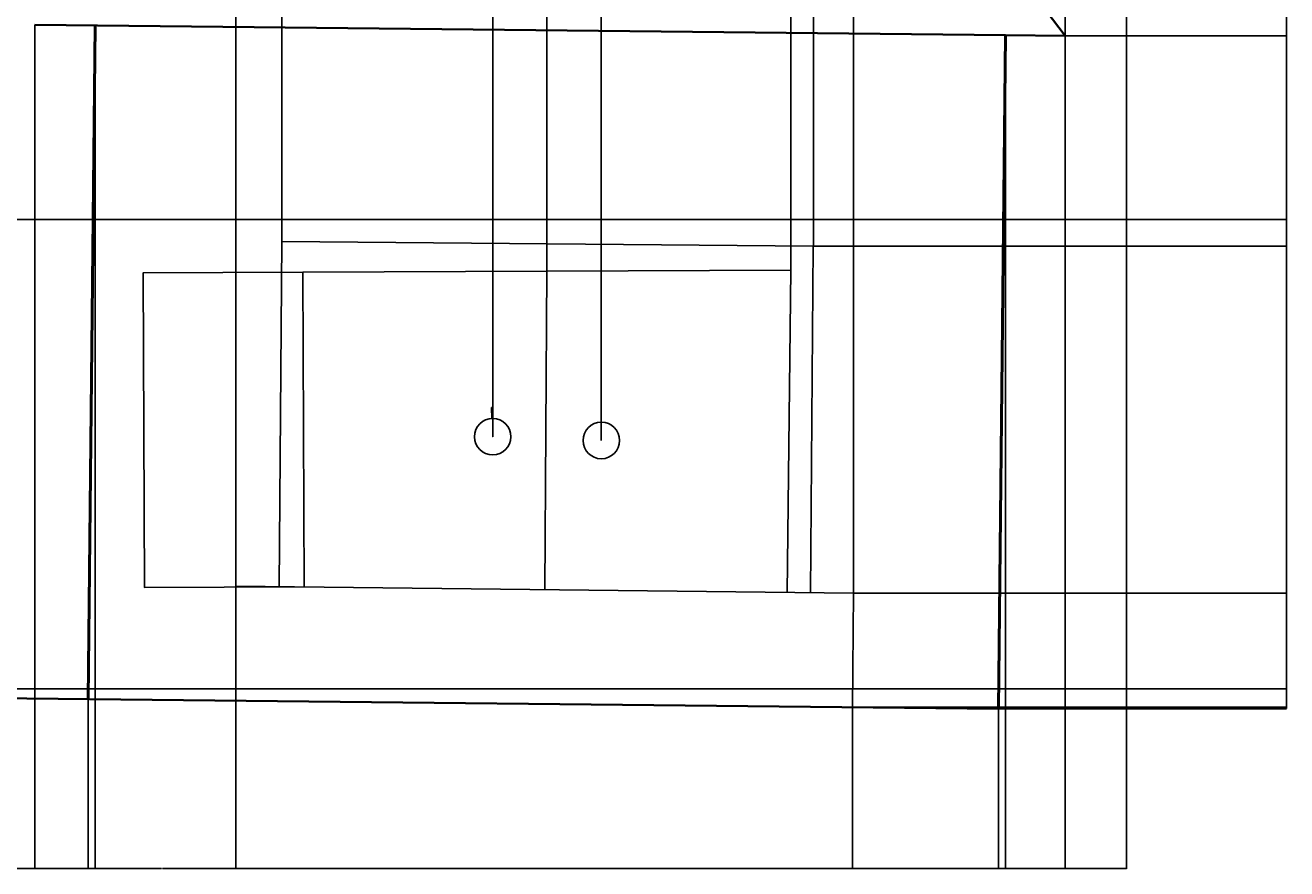
# Model space of a CAD drawing. Units: millimetres. Extents: x 1119 to 4262, y 854 to 2737.
# Tile 4 of 5: x 3118 to 4262, y 854 to 1620. Entities that reach past the tile are written whole.
import ezdxf

# ---------------------------------------------------------------- set-up
doc = ezdxf.new("R2010")
doc.units = ezdxf.units.MM
for name, color, linetype, lineweight in [('A-ANNO-DIMS', 2, 'Continuous', 18), ('A-DOOR', 3, 'Continuous', 25), ('A-ELEV', 8, 'Continuous', 35), ('A-FLOR-STRS', 6, 'Continuous', 25), ('A-ROOF', 1, 'Continuous', 35), ('A-WALL', 7, 'Continuous', 50)]:
    doc.layers.add(name, color=color, linetype=linetype, lineweight=lineweight)
doc.styles.get("Standard").update_dxf_attribs({"font": 'arial.ttf'})
doc.dimstyles.get("Standard").update_dxf_attribs({"dimtxt": 0.18, "dimasz": 0.18, "dimexe": 0.18, "dimexo": 0.0625, "dimgap": 0.09, "dimtad": 0, "dimtih": 1, "dimtoh": 1, "dimdec": 4, "dimzin": 0, "dimdsep": 46, "dimtxsty": 'Standard', "dimcen": 0.09, "dimadec": 0, "dimazin": 0, "dimtfac": 1, "dimtdec": 4, "dimtofl": 0, "dimtmove": 0, "dimatfit": 3, "dimfxl": 1, "dimtolj": 1, "dimtzin": 0, "dimarcsym": 0})

# ---------------------------------------------------------------- blocks, each defined once
blk = doc.blocks.new('*D9')
at = {"layer": 'A-ANNO-DIMS', "color": 0, "lineweight": -2, "transparency": 16777216}
for p, q in [((3099.2, 1180.2), (3099.2, 854.2)), ((3174.6, 1008), (3174.6, 854.2)), ((3099.4, 854.4), (3136.5, 854.4)), ((3174.4, 854.4), (3137.3, 854.4))]:
    blk.add_line(p, q, dxfattribs=at)
at = {"layer": 'A-ANNO-DIMS', "color": 0, "transparency": 16777216}
for points in [[(3099.4, 854.4), (3099.4, 854.3), (3099.2, 854.4)], [(3174.4, 854.4), (3174.4, 854.3), (3174.6, 854.4)]]:
    blk.add_solid(points, dxfattribs=at)
at = {"layer": 'Defpoints', "color": 0, "transparency": 16777216}
for p in [(3099.2, 1180.2), (3174.6, 1008.1), (3174.6, 854.4)]:
    blk.add_point(p, dxfattribs=at)
at = {"layer": 'A-ANNO-DIMS', "color": 0, "transparency": 16777216, "insert": (3136.9, 854.4), "char_height": 0.18, "attachment_point": 5}
blk.add_mtext('\\A1;75.38', dxfattribs=at)
blk = doc.blocks.new('*D10')
at = {"layer": 'A-ANNO-DIMS', "color": 0, "lineweight": -2, "transparency": 16777216}
for p, q in [((3174.6, 1008), (3174.6, 854.2)), ((3308.7, 1006.6), (3308.7, 854.2)), ((3174.7, 854.4), (3241.2, 854.4)), ((3308.5, 854.4), (3242.1, 854.4))]:
    blk.add_line(p, q, dxfattribs=at)
at = {"layer": 'A-ANNO-DIMS', "color": 0, "transparency": 16777216}
for points in [[(3174.7, 854.4), (3174.7, 854.3), (3174.6, 854.4)], [(3308.5, 854.4), (3308.5, 854.3), (3308.7, 854.4)]]:
    blk.add_solid(points, dxfattribs=at)
at = {"layer": 'Defpoints', "color": 0, "transparency": 16777216}
for p in [(3174.6, 1008.1), (3308.7, 1006.7), (3308.7, 854.4)]:
    blk.add_point(p, dxfattribs=at)
at = {"layer": 'A-ANNO-DIMS', "color": 0, "transparency": 16777216, "insert": (3241.6, 854.4), "char_height": 0.18, "attachment_point": 5}
blk.add_mtext('\\A1;134.12', dxfattribs=at)
blk = doc.blocks.new('*D11')
at = {"layer": 'A-ANNO-DIMS', "color": 0, "lineweight": -2, "transparency": 16777216}
for p, q in [((3308.7, 1006.6), (3308.7, 854.2)), ((4000.5, 999.3), (4000.5, 854.2)), ((3308.9, 854.4), (3654.2, 854.4)), ((4000.4, 854.4), (3655, 854.4))]:
    blk.add_line(p, q, dxfattribs=at)
at = {"layer": 'A-ANNO-DIMS', "color": 0, "transparency": 16777216}
for points in [[(3308.9, 854.4), (3308.9, 854.3), (3308.7, 854.4)], [(4000.4, 854.4), (4000.4, 854.3), (4000.5, 854.4)]]:
    blk.add_solid(points, dxfattribs=at)
at = {"layer": 'Defpoints', "color": 0, "transparency": 16777216}
for p in [(3308.7, 1006.7), (4000.5, 999.4), (4000.5, 854.4)]:
    blk.add_point(p, dxfattribs=at)
at = {"layer": 'A-ANNO-DIMS', "color": 0, "transparency": 16777216, "insert": (3654.6, 854.4), "char_height": 0.18, "attachment_point": 5}
blk.add_mtext('\\A1;691.9', dxfattribs=at)
blk = doc.blocks.new('*D12')
at = {"layer": 'A-ANNO-DIMS', "color": 0, "lineweight": -2, "transparency": 16777216}
for p, q in [((4116.8, 2249.7), (4116.8, 854.2)), ((4000.5, 999.3), (4000.5, 854.2)), ((4000.7, 854.4), (4058.2, 854.4)), ((4116.6, 854.4), (4059.1, 854.4))]:
    blk.add_line(p, q, dxfattribs=at)
at = {"layer": 'A-ANNO-DIMS', "color": 0, "transparency": 16777216}
for points in [[(4000.7, 854.4), (4000.7, 854.3), (4000.5, 854.4)], [(4116.6, 854.4), (4116.6, 854.3), (4116.8, 854.4)]]:
    blk.add_solid(points, dxfattribs=at)
at = {"layer": 'Defpoints', "color": 0, "transparency": 16777216}
for p in [(4116.8, 2249.7), (4000.5, 999.4), (4116.8, 854.4)]:
    blk.add_point(p, dxfattribs=at)
at = {"layer": 'A-ANNO-DIMS', "color": 0, "transparency": 16777216, "insert": (4058.7, 854.4), "char_height": 0.18, "attachment_point": 5}
blk.add_mtext('\\A1;116.25', dxfattribs=at)
blk = doc.blocks.new('*D13')
at = {"layer": 'A-ANNO-DIMS', "color": 0, "lineweight": -2, "transparency": 16777216}
for p, q in [((1264.4, 1028.3), (1264.4, 2737.1)), ((1264.5, 2737), (2690.1, 2737)), ((4116.6, 2737), (2691, 2737)), ((4116.8, 2249.8), (4116.8, 2737.1))]:
    blk.add_line(p, q, dxfattribs=at)
at = {"layer": 'A-ANNO-DIMS', "color": 0, "transparency": 16777216}
for points in [[(1264.5, 2737), (1264.5, 2736.9), (1264.4, 2737)], [(4116.6, 2737), (4116.6, 2736.9), (4116.8, 2737)]]:
    blk.add_solid(points, dxfattribs=at)
at = {"layer": 'Defpoints', "color": 0, "transparency": 16777216}
for p in [(4116.8, 2737), (4116.8, 2249.7), (1264.4, 1028.2)]:
    blk.add_point(p, dxfattribs=at)
at = {"layer": 'A-ANNO-DIMS', "color": 0, "transparency": 16777216, "insert": (2690.6, 2737), "char_height": 0.18, "attachment_point": 5}
blk.add_mtext('\\A1;2852.4', dxfattribs=at)
blk = doc.blocks.new('*D37')
at = {"layer": 'A-ANNO-DIMS', "color": 0, "lineweight": -2, "transparency": 16777216}
for p, q in [((3869.2, 1104.3), (4262, 1104.3)), ((4261.8, 1104.1), (4261.8, 1052)), ((4261.8, 999.5), (4261.8, 1051.7)), ((4000.6, 999.4), (4262, 999.4))]:
    blk.add_line(p, q, dxfattribs=at)
at = {"layer": 'A-ANNO-DIMS', "color": 0, "transparency": 16777216}
for points in [[(4261.8, 1104.1), (4261.8, 1104.1), (4261.8, 1104.3)], [(4261.8, 999.5), (4261.8, 999.5), (4261.8, 999.4)]]:
    blk.add_solid(points, dxfattribs=at)
at = {"layer": 'Defpoints', "color": 0, "transparency": 16777216}
for p in [(3869.1, 1104.3), (4261.8, 1104.3), (4000.5, 999.4)]:
    blk.add_point(p, dxfattribs=at)
at = {"layer": 'A-ANNO-DIMS', "color": 0, "transparency": 16777216, "insert": (4261.8, 1051.8), "char_height": 0.18, "attachment_point": 5}
blk.add_mtext('\\A1;104.95', dxfattribs=at)
blk = doc.blocks.new('*D38')
at = {"layer": 'A-ANNO-DIMS', "color": 0, "lineweight": -2, "transparency": 16777216}
for p, q in [((4061.2, 1610.2), (4262, 1610.2)), ((4261.8, 1610.1), (4261.8, 1357.5)), ((4261.8, 1104.5), (4261.8, 1357.1)), ((3869.2, 1104.3), (4262, 1104.3))]:
    blk.add_line(p, q, dxfattribs=at)
at = {"layer": 'A-ANNO-DIMS', "color": 0, "transparency": 16777216}
for points in [[(4261.8, 1610.1), (4261.8, 1610.1), (4261.8, 1610.2)], [(4261.8, 1104.5), (4261.8, 1104.5), (4261.8, 1104.3)]]:
    blk.add_solid(points, dxfattribs=at)
at = {"layer": 'Defpoints', "color": 0, "transparency": 16777216}
for p in [(4061.1, 1610.2), (4261.8, 1610.2), (3869.1, 1104.3)]:
    blk.add_point(p, dxfattribs=at)
at = {"layer": 'A-ANNO-DIMS', "color": 0, "transparency": 16777216, "insert": (4261.8, 1357.3), "char_height": 0.18, "attachment_point": 5}
blk.add_mtext('\\A1;505.9', dxfattribs=at)
blk = doc.blocks.new('*D39')
at = {"layer": 'A-ANNO-DIMS', "color": 0, "lineweight": -2, "transparency": 16777216}
for p, q in [((3962.6, 1739.8), (4262, 1739.8)), ((4261.8, 1739.6), (4261.8, 1675.2)), ((4261.8, 1610.4), (4261.8, 1674.8)), ((4061.2, 1610.2), (4262, 1610.2))]:
    blk.add_line(p, q, dxfattribs=at)
at = {"layer": 'A-ANNO-DIMS', "color": 0, "transparency": 16777216}
for points in [[(4261.8, 1739.6), (4261.8, 1739.6), (4261.8, 1739.8)], [(4261.8, 1610.4), (4261.8, 1610.4), (4261.8, 1610.2)]]:
    blk.add_solid(points, dxfattribs=at)
at = {"layer": 'Defpoints', "color": 0, "transparency": 16777216}
for p in [(3962.6, 1739.8), (4261.8, 1739.8), (4061.1, 1610.2)]:
    blk.add_point(p, dxfattribs=at)
at = {"layer": 'A-ANNO-DIMS', "color": 0, "transparency": 16777216, "insert": (4261.8, 1675), "char_height": 0.18, "attachment_point": 5}
blk.add_mtext('\\A1;129.59', dxfattribs=at)
blk = doc.blocks.new('*D64')
at = {"layer": 'A-ANNO-DIMS', "color": 0, "lineweight": -2, "transparency": 16777216}
for p, q in [((3962.6, 1739.9), (3962.6, 2737.1)), ((3962.7, 2737), (4011.4, 2737)), ((4060.9, 2737), (4012.2, 2737)), ((4061.1, 1610.3), (4061.1, 2737.1))]:
    blk.add_line(p, q, dxfattribs=at)
at = {"layer": 'A-ANNO-DIMS', "color": 0, "transparency": 16777216}
for points in [[(3962.7, 2737), (3962.7, 2736.9), (3962.6, 2737)], [(4060.9, 2737), (4060.9, 2736.9), (4061.1, 2737)]]:
    blk.add_solid(points, dxfattribs=at)
at = {"layer": 'Defpoints', "color": 0, "transparency": 16777216}
for p in [(4061.1, 2737), (3962.6, 1739.8), (4061.1, 1610.2)]:
    blk.add_point(p, dxfattribs=at)
at = {"layer": 'A-ANNO-DIMS', "color": 0, "transparency": 16777216, "insert": (4011.8, 2737), "char_height": 0.18, "attachment_point": 5}
blk.add_mtext('\\A1;98.53', dxfattribs=at)
blk = doc.blocks.new('*D65')
at = {"layer": 'A-ANNO-DIMS', "color": 0, "lineweight": -2, "transparency": 16777216}
for p, q in [((3126.3, 1620), (3126.3, 854.2)), ((3181, 1619.4), (3181, 854.2)), ((3126.4, 854.4), (3153.2, 854.4)), ((3180.8, 854.4), (3154, 854.4))]:
    blk.add_line(p, q, dxfattribs=at)
at = {"layer": 'A-ANNO-DIMS', "color": 0, "transparency": 16777216}
for points in [[(3126.4, 854.4), (3126.4, 854.3), (3126.3, 854.4)], [(3180.8, 854.4), (3180.8, 854.3), (3181, 854.4)]]:
    blk.add_solid(points, dxfattribs=at)
at = {"layer": 'Defpoints', "color": 0, "transparency": 16777216}
for p in [(3126.3, 1620.1), (3181, 1619.5), (3181, 854.4)]:
    blk.add_point(p, dxfattribs=at)
at = {"layer": 'A-ANNO-DIMS', "color": 0, "transparency": 16777216, "insert": (3153.6, 854.4), "char_height": 0.18, "attachment_point": 5}
blk.add_mtext('\\A1;54.74', dxfattribs=at)
blk = doc.blocks.new('*D66')
at = {"layer": 'A-ANNO-DIMS', "color": 0, "lineweight": -2, "transparency": 16777216}
for p, q in [((4007, 1610.7), (4007, 854.2)), ((4061.1, 1610.2), (4061.1, 854.2)), ((4007.2, 854.4), (4033.7, 854.4)), ((4060.9, 854.4), (4034.3, 854.4))]:
    blk.add_line(p, q, dxfattribs=at)
at = {"layer": 'A-ANNO-DIMS', "color": 0, "transparency": 16777216}
for points in [[(4007.2, 854.4), (4007.2, 854.3), (4007, 854.4)], [(4060.9, 854.4), (4060.9, 854.3), (4061.1, 854.4)]]:
    blk.add_solid(points, dxfattribs=at)
at = {"layer": 'Defpoints', "color": 0, "transparency": 16777216}
for p in [(4007, 1610.8), (4061.1, 1610.2), (4061.1, 854.4)]:
    blk.add_point(p, dxfattribs=at)
at = {"layer": 'A-ANNO-DIMS', "color": 0, "transparency": 16777216, "insert": (4034, 854.4), "char_height": 0.18, "attachment_point": 5}
blk.add_mtext('\\A1;54.1', dxfattribs=at)
blk = doc.blocks.new('*D78')
at = {"layer": 'A-ANNO-DIMS', "color": 0, "lineweight": -2, "transparency": 16777216}
for p, q in [((2297.6, 1443.4), (4262, 1443.4)), ((4261.8, 1443.2), (4261.8, 1230.6)), ((4261.8, 1017.5), (4261.8, 1230.2)), ((2293.1, 1017.4), (4262, 1017.4))]:
    blk.add_line(p, q, dxfattribs=at)
at = {"layer": 'A-ANNO-DIMS', "color": 0, "transparency": 16777216}
for points in [[(4261.8, 1443.2), (4261.8, 1443.2), (4261.8, 1443.4)], [(4261.8, 1017.5), (4261.8, 1017.5), (4261.8, 1017.4)]]:
    blk.add_solid(points, dxfattribs=at)
at = {"layer": 'Defpoints', "color": 0, "transparency": 16777216}
for p in [(2297.6, 1443.4), (4261.8, 1443.4), (2293.1, 1017.4)]:
    blk.add_point(p, dxfattribs=at)
at = {"layer": 'A-ANNO-DIMS', "color": 0, "transparency": 16777216, "insert": (4261.8, 1230.4), "char_height": 0.18, "attachment_point": 5}
blk.add_mtext('\\A1;426.06', dxfattribs=at)
blk = doc.blocks.new('*D80')
at = {"layer": 'A-ANNO-DIMS', "color": 0, "lineweight": -2, "transparency": 16777216}
for p, q in [((3308.7, 1006.6), (3308.7, 854.2)), ((3868, 1000.7), (3868, 854.2)), ((3308.9, 854.4), (3588, 854.4)), ((3867.8, 854.4), (3588.7, 854.4))]:
    blk.add_line(p, q, dxfattribs=at)
at = {"layer": 'A-ANNO-DIMS', "color": 0, "transparency": 16777216}
for points in [[(3308.9, 854.4), (3308.9, 854.3), (3308.7, 854.4)], [(3867.8, 854.4), (3867.8, 854.3), (3868, 854.4)]]:
    blk.add_solid(points, dxfattribs=at)
at = {"layer": 'Defpoints', "color": 0, "transparency": 16777216}
for p in [(3308.7, 1006.7), (3868, 1000.8), (3868, 854.4)]:
    blk.add_point(p, dxfattribs=at)
at = {"layer": 'A-ANNO-DIMS', "color": 0, "transparency": 16777216, "insert": (3588.3, 854.4), "char_height": 0.18, "attachment_point": 5}
blk.add_mtext('\\A1;559.4', dxfattribs=at)
blk = doc.blocks.new('*D81')
at = {"layer": 'A-ANNO-DIMS', "color": 0, "lineweight": -2, "transparency": 16777216}
for p, q in [((3308.6, 1110.8), (3308.6, 2737.1)), ((3308.8, 2737), (3329.2, 2737)), ((3350.3, 2737), (3329.9, 2737)), ((3350.4, 1423.5), (3350.4, 2737.1))]:
    blk.add_line(p, q, dxfattribs=at)
at = {"layer": 'A-ANNO-DIMS', "color": 0, "transparency": 16777216}
for points in [[(3308.8, 2737), (3308.8, 2736.9), (3308.6, 2737)], [(3350.3, 2737), (3350.3, 2736.9), (3350.4, 2737)]]:
    blk.add_solid(points, dxfattribs=at)
at = {"layer": 'Defpoints', "color": 0, "transparency": 16777216}
for p in [(3350.4, 2737), (3350.4, 1423.4), (3308.6, 1110.7)]:
    blk.add_point(p, dxfattribs=at)
at = {"layer": 'A-ANNO-DIMS', "color": 0, "transparency": 16777216, "insert": (3329.5, 2737), "char_height": 0.18, "attachment_point": 5}
blk.add_mtext('\\A1;41.8', dxfattribs=at)
blk = doc.blocks.new('*D82')
at = {"layer": 'A-ANNO-DIMS', "color": 0, "lineweight": -2, "transparency": 16777216}
for p, q in [((3350.4, 1423.5), (3350.4, 2737.1)), ((3350.6, 2737), (3470.2, 2737)), ((3590.6, 2737), (3471, 2737)), ((3590.8, 1396.6), (3590.8, 2737.1))]:
    blk.add_line(p, q, dxfattribs=at)
at = {"layer": 'A-ANNO-DIMS', "color": 0, "transparency": 16777216}
for points in [[(3350.6, 2737), (3350.6, 2736.9), (3350.4, 2737)], [(3590.6, 2737), (3590.6, 2736.9), (3590.8, 2737)]]:
    blk.add_solid(points, dxfattribs=at)
at = {"layer": 'Defpoints', "color": 0, "transparency": 16777216}
for p in [(3590.8, 2737), (3350.4, 1423.4), (3590.8, 1396.6)]:
    blk.add_point(p, dxfattribs=at)
at = {"layer": 'A-ANNO-DIMS', "color": 0, "transparency": 16777216, "insert": (3470.6, 2737), "char_height": 0.18, "attachment_point": 5}
blk.add_mtext('\\A1;240.4', dxfattribs=at)
blk = doc.blocks.new('*D83')
at = {"layer": 'A-ANNO-DIMS', "color": 0, "lineweight": -2, "transparency": 16777216}
for p, q in [((3590.8, 1396.6), (3590.8, 2737.1)), ((3591, 2737), (3701.1, 2737)), ((3812.1, 2737), (3702, 2737)), ((3812.3, 1397.6), (3812.3, 2737.1))]:
    blk.add_line(p, q, dxfattribs=at)
at = {"layer": 'A-ANNO-DIMS', "color": 0, "transparency": 16777216}
for points in [[(3591, 2737), (3591, 2736.9), (3590.8, 2737)], [(3812.1, 2737), (3812.1, 2736.9), (3812.3, 2737)]]:
    blk.add_solid(points, dxfattribs=at)
at = {"layer": 'Defpoints', "color": 0, "transparency": 16777216}
for p in [(3812.3, 2737), (3590.8, 1396.6), (3812.3, 1397.5)]:
    blk.add_point(p, dxfattribs=at)
at = {"layer": 'A-ANNO-DIMS', "color": 0, "transparency": 16777216, "insert": (3701.5, 2737), "char_height": 0.18, "attachment_point": 5}
blk.add_mtext('\\A1;221.45', dxfattribs=at)
blk = doc.blocks.new('*D84')
at = {"layer": 'A-ANNO-DIMS', "color": 0, "lineweight": -2, "transparency": 16777216}
for p, q in [((3812.3, 1397.6), (3812.3, 2737.1)), ((3812.5, 2737), (3822, 2737)), ((3832.4, 2737), (3822.8, 2737)), ((3832.6, 1419.5), (3832.6, 2737.1))]:
    blk.add_line(p, q, dxfattribs=at)
at = {"layer": 'A-ANNO-DIMS', "color": 0, "transparency": 16777216}
for points in [[(3812.5, 2737), (3812.5, 2736.9), (3812.3, 2737)], [(3832.4, 2737), (3832.4, 2736.9), (3832.6, 2737)]]:
    blk.add_solid(points, dxfattribs=at)
at = {"layer": 'Defpoints', "color": 0, "transparency": 16777216}
for p in [(3832.6, 2737), (3832.6, 1419.4), (3812.3, 1397.5)]:
    blk.add_point(p, dxfattribs=at)
at = {"layer": 'A-ANNO-DIMS', "color": 0, "transparency": 16777216, "insert": (3822.4, 2737), "char_height": 0.18, "attachment_point": 5}
blk.add_mtext('\\A1;20.32', dxfattribs=at)
blk = doc.blocks.new('*D85')
at = {"layer": 'A-ANNO-DIMS', "color": 0, "lineweight": -2, "transparency": 16777216}
for p, q in [((3832.6, 1419.5), (3832.6, 2737.1)), ((3832.8, 2737), (3850.4, 2737)), ((3868.9, 2737), (3851.3, 2737)), ((3869.1, 1104.4), (3869.1, 2737.1))]:
    blk.add_line(p, q, dxfattribs=at)
at = {"layer": 'A-ANNO-DIMS', "color": 0, "transparency": 16777216}
for points in [[(3832.8, 2737), (3832.8, 2736.9), (3832.6, 2737)], [(3868.9, 2737), (3868.9, 2736.9), (3869.1, 2737)]]:
    blk.add_solid(points, dxfattribs=at)
at = {"layer": 'Defpoints', "color": 0, "transparency": 16777216}
for p in [(3869.1, 2737), (3832.6, 1419.4), (3869.1, 1104.3)]:
    blk.add_point(p, dxfattribs=at)
at = {"layer": 'A-ANNO-DIMS', "color": 0, "transparency": 16777216, "insert": (3850.9, 2737), "char_height": 0.18, "attachment_point": 5}
blk.add_mtext('\\A1;36.526', dxfattribs=at)
blk = doc.blocks.new('*D86')
at = {"layer": 'A-ANNO-DIMS', "color": 0, "lineweight": -2, "transparency": 16777216}
for p, q in [((3541.7, 1246.4), (3541.7, 2737.1)), ((3541.9, 2737), (3590.6, 2737)), ((3640.1, 2737), (3591.4, 2737)), ((3640.2, 1243), (3640.2, 2737.1))]:
    blk.add_line(p, q, dxfattribs=at)
at = {"layer": 'A-ANNO-DIMS', "color": 0, "transparency": 16777216}
for points in [[(3541.9, 2737), (3541.9, 2736.9), (3541.7, 2737)], [(3640.1, 2737), (3640.1, 2736.9), (3640.2, 2737)]]:
    blk.add_solid(points, dxfattribs=at)
at = {"layer": 'Defpoints', "color": 0, "transparency": 16777216}
for p in [(3640.2, 2737), (3541.7, 1246.4), (3640.2, 1242.9)]:
    blk.add_point(p, dxfattribs=at)
at = {"layer": 'A-ANNO-DIMS', "color": 0, "transparency": 16777216, "insert": (3591, 2737), "char_height": 0.18, "attachment_point": 5}
blk.add_mtext('\\A1;98.55', dxfattribs=at)
blk = doc.blocks.new('*D87')
at = {"layer": 'A-ANNO-DIMS', "color": 0, "lineweight": -2, "transparency": 16777216}
for p, q in [((3369.3, 1395.6), (3224.2, 1395)), ((3224.4, 1394.9), (3225, 1252.4)), ((3225.6, 1109.6), (3225, 1252)), ((3370.5, 1110), (3225.4, 1109.4))]:
    blk.add_line(p, q, dxfattribs=at)
at = {"layer": 'A-ANNO-DIMS', "color": 0, "transparency": 16777216}
for points in [[(3224.4, 1394.9), (3224.3, 1394.9), (3224.4, 1395)], [(3225.6, 1109.6), (3225.5, 1109.6), (3225.6, 1109.4)]]:
    blk.add_solid(points, dxfattribs=at)
at = {"layer": 'Defpoints', "color": 0, "transparency": 16777216}
for p in [(3224.4, 1395), (3369.4, 1395.6), (3370.6, 1110)]:
    blk.add_point(p, dxfattribs=at)
at = {"layer": 'A-ANNO-DIMS', "color": 0, "transparency": 16777216, "insert": (3225, 1252.2), "char_height": 0.18, "attachment_point": 5}
blk.add_mtext('\\A1;285.66', dxfattribs=at)
blk = doc.blocks.new('*D88')
at = {"layer": 'A-ANNO-DIMS', "color": 0, "lineweight": -2, "transparency": 16777216}
for p, q in [((3869.2, 1104.3), (4262, 1104.3)), ((4261.8, 1104.1), (4261.8, 1052.7)), ((4261.8, 1000.9), (4261.8, 1052.3)), ((3868.1, 1000.8), (4262, 1000.8))]:
    blk.add_line(p, q, dxfattribs=at)
at = {"layer": 'A-ANNO-DIMS', "color": 0, "transparency": 16777216}
for points in [[(4261.8, 1104.1), (4261.8, 1104.1), (4261.8, 1104.3)], [(4261.8, 1000.9), (4261.8, 1000.9), (4261.8, 1000.8)]]:
    blk.add_solid(points, dxfattribs=at)
at = {"layer": 'Defpoints', "color": 0, "transparency": 16777216}
for p in [(3869.1, 1104.3), (4261.8, 1104.3), (3868, 1000.8)]:
    blk.add_point(p, dxfattribs=at)
at = {"layer": 'A-ANNO-DIMS', "color": 0, "transparency": 16777216, "insert": (4261.8, 1052.5), "char_height": 0.18, "attachment_point": 5}
blk.add_mtext('\\A1;103.55', dxfattribs=at)
blk = doc.blocks.new('*D89')
at = {"layer": 'A-ANNO-DIMS', "color": 0, "lineweight": -2, "transparency": 16777216}
for p, q in [((3832.7, 1419.4), (4262, 1419.4)), ((4261.8, 1419.2), (4261.8, 1262)), ((4261.8, 1104.5), (4261.8, 1261.7)), ((3869.2, 1104.3), (4262, 1104.3))]:
    blk.add_line(p, q, dxfattribs=at)
at = {"layer": 'A-ANNO-DIMS', "color": 0, "transparency": 16777216}
for points in [[(4261.8, 1419.2), (4261.8, 1419.2), (4261.8, 1419.4)], [(4261.8, 1104.5), (4261.8, 1104.5), (4261.8, 1104.3)]]:
    blk.add_solid(points, dxfattribs=at)
at = {"layer": 'Defpoints', "color": 0, "transparency": 16777216}
for p in [(3832.6, 1419.4), (4261.8, 1419.4), (3869.1, 1104.3)]:
    blk.add_point(p, dxfattribs=at)
at = {"layer": 'A-ANNO-DIMS', "color": 0, "transparency": 16777216, "insert": (4261.8, 1261.9), "char_height": 0.18, "attachment_point": 5}
blk.add_mtext('\\A1;315.1', dxfattribs=at)
blk = doc.blocks.new('*D91')
at = {"layer": 'A-ANNO-DIMS', "color": 0, "lineweight": -2, "transparency": 16777216}
for p, q in [((3540.4, 1272.7), (3540.6, 1272.7)), ((3540.6, 1272.7), (3541, 1263)), ((3541.6, 1246.4), (3541.8, 1246.4)), ((3541.7, 1246.3), (3541.7, 1246.4))]:
    blk.add_line(p, q, dxfattribs=at)
at = {"layer": 'A-ANNO-DIMS', "color": 0, "transparency": 16777216}
blk.add_solid([(3541, 1263), (3541, 1263), (3541, 1262.8)], dxfattribs=at)
at = {"layer": 'Defpoints', "color": 0, "transparency": 16777216}
for p in [(3541, 1262.8), (3542.4, 1229.9)]:
    blk.add_point(p, dxfattribs=at)
at = {"layer": 'A-ANNO-DIMS', "color": 0, "transparency": 16777216, "insert": (3539.7, 1272.7), "char_height": 0.18, "attachment_point": 5}
blk.add_mtext('\\A1;2X ∅32.98', dxfattribs=at)

msp = doc.modelspace()

# ---------------------------------------------------------------- linework, layer by layer
at = {"layer": 'A-DOOR'}
for p, q in [((3347.8602, 1110.2436), (3350.4459, 1423.3892)), ((3350.4459, 1423.3892), (3832.5892, 1419.4082)), ((3832.5892, 1419.4082), (3829.9911, 1104.7538)), ((3369.3754, 1395.6431), (3812.2711, 1397.4995)), ((3590.8232, 1396.5713), (3588.8816, 1107.4992)), ((3812.2711, 1397.4995), (3808.9405, 1104.9935)), ((3370.5727, 1109.985), (3369.3754, 1395.6431))]:
    msp.add_line(p, q, dxfattribs=at)
for centre, radius in [((3541.6938, 1246.3571), 16.4912), ((3640.2453, 1242.9086), 16.5944)]:
    msp.add_circle(centre, radius, dxfattribs=at)
at = {"layer": 'A-ELEV'}
msp.add_line((1264.3595, 1028.2021), (4000.5454, 999.3572), dxfattribs=at)
at = {"layer": 'A-FLOR-STRS'}
for p, q in [((3308.6716, 1006.651), (3308.6482, 1110.6901)), ((3308.6482, 1110.6901), (3869.1151, 1104.3083)), ((3869.1151, 1104.3083), (3868.0234, 1000.7543))]:
    msp.add_line(p, q, dxfattribs=at)
at = {"layer": 'A-ROOF'}
for p, q in [((3962.5635, 1739.8164), (4061.0895, 1610.2307)), ((4006.9912, 1610.801), (3126.2541, 1620.0857)), ((4006.9912, 1610.801), (4061.0895, 1610.2307))]:
    msp.add_line(p, q, dxfattribs=at)
at = {"layer": 'A-WALL'}
for p, q in [((3180.996, 1619.5086), (3174.5502, 1008.0649)), ((4000.5454, 999.3572), (4006.9912, 1610.801))]:
    msp.add_line(p, q, dxfattribs=at)

# ---------------------------------------------------------------- dimensions: what is measured, and where the dimension line sits
at = {"layer": 'A-ANNO-DIMS'}
for base, p1, p2, override, picture, middle in [((4116.7957, 2736.9672), (1264.3595, 1028.2021), (4116.7957, 2249.7378), {"dimdec": 1, "dimlfac": 1, "dimrnd": 0, "dimzin": 0, "dimdsep": 46, "dimlunit": 2}, '*D13', (2690.5776, 2736.9672)), ((3350.4459, 2736.9672), (3308.6482, 1110.6901), (3350.4459, 1423.3892), {"dimdec": 1, "dimlfac": 1, "dimrnd": 0, "dimzin": 0, "dimdsep": 46, "dimlunit": 2}, '*D81', (3329.547, 2736.9672)), ((3590.8232, 2736.9672), (3350.4459, 1423.3892), (3590.8232, 1396.5713), {"dimdec": 1, "dimlfac": 1, "dimrnd": 0, "dimzin": 0, "dimdsep": 46, "dimlunit": 2}, '*D82', (3470.6345, 2736.9672)), ((3640.2453, 2736.9672), (3541.6938, 1246.3571), (3640.2453, 1242.9086), {"dimdec": 2, "dimlfac": 1, "dimrnd": 0, "dimzin": 0, "dimdsep": 46, "dimlunit": 2}, '*D86', (3590.9696, 2736.9672)), ((3812.2711, 2736.9672), (3590.8232, 1396.5713), (3812.2711, 1397.4995), {"dimdec": 2, "dimlfac": 1, "dimrnd": 0, "dimzin": 0, "dimdsep": 46, "dimlunit": 2}, '*D83', (3701.5472, 2736.9672)), ((3832.5892, 2736.9672), (3812.2711, 1397.4995), (3832.5892, 1419.4082), {"dimdec": 2, "dimlfac": 1, "dimrnd": 0, "dimzin": 0, "dimdsep": 46, "dimlunit": 2}, '*D84', (3822.4302, 2736.9672)), ((3869.1151, 2736.9672), (3832.5892, 1419.4082), (3869.1151, 1104.3083), {"dimdec": 3, "dimlfac": 1, "dimrnd": 0, "dimzin": 0, "dimdsep": 46, "dimlunit": 2}, '*D85', (3850.8521, 2736.9672)), ((4061.0895, 2736.9672), (3962.5635, 1739.8164), (4061.0895, 1610.2307), {"dimdec": 2, "dimlfac": 1, "dimrnd": 0, "dimzin": 0, "dimdsep": 46, "dimlunit": 2}, '*D64', (4011.8265, 2736.9672)), ((4116.7957, 854.3572), (4000.5454, 999.3572), (4116.7957, 2249.7378), {"dimdec": 2, "dimlfac": 1, "dimrnd": 0, "dimzin": 0, "dimdsep": 46, "dimlunit": 2}, '*D12', (4058.6705, 854.3572)), ((3180.996, 854.3572), (3126.2541, 1620.0857), (3180.996, 1619.5086), {"dimdec": 2, "dimlfac": 1, "dimrnd": 0, "dimzin": 0, "dimdsep": 46, "dimlunit": 2}, '*D65', (3153.6251, 854.3572)), ((4061.0895, 854.3572), (4006.9912, 1610.801), (4061.0895, 1610.2307), {"dimdec": 1, "dimlfac": 1, "dimrnd": 0, "dimzin": 0, "dimdsep": 46, "dimlunit": 2}, '*D66', (4034.0404, 854.3572)), ((3174.5502, 854.3572), (3099.1711, 1180.2494), (3174.5502, 1008.0649), {"dimdec": 2, "dimlfac": 1, "dimrnd": 0, "dimzin": 0, "dimdsep": 46, "dimlunit": 2}, '*D9', (3136.8606, 854.3572)), ((3308.6716, 854.3572), (3174.5502, 1008.0649), (3308.6716, 1006.651), {"dimdec": 2, "dimlfac": 1, "dimrnd": 0, "dimzin": 0, "dimdsep": 46, "dimlunit": 2}, '*D10', (3241.6109, 854.3572)), ((4000.5454, 854.3572), (3308.6716, 1006.651), (4000.5454, 999.3572), {"dimdec": 1, "dimlfac": 1, "dimrnd": 0, "dimzin": 0, "dimdsep": 46, "dimlunit": 2}, '*D11', (3654.6085, 854.3572)), ((3868.0234, 854.3572), (3308.6716, 1006.651), (3868.0234, 1000.7543), {"dimdec": 1, "dimlfac": 1, "dimrnd": 0, "dimzin": 0, "dimdsep": 46, "dimlunit": 2}, '*D80', (3588.3475, 854.3572))]:
    dim = msp.add_linear_dim(base=base, p1=p1, p2=p2, dimstyle='Standard', override=override, dxfattribs=at)
    dim.commit()
    dim.dimension.update_dxf_attribs({"geometry": picture, "text_midpoint": middle})
for base, p1, p2, angle, override, picture, middle in [((4261.7957, 1739.8164), (4061.0895, 1610.2307), (3962.5635, 1739.8164), 90, {"dimdec": 2, "dimlfac": 1, "dimrnd": 0, "dimzin": 0, "dimdsep": 46, "dimlunit": 2}, '*D39', (4261.7957, 1675.0236)), ((4261.7957, 1610.2307), (3869.1151, 1104.3083), (4061.0895, 1610.2307), 90, {"dimdec": 1, "dimlfac": 1, "dimrnd": 0, "dimzin": 0, "dimdsep": 46, "dimlunit": 2}, '*D38', (4261.7957, 1357.2695)), ((4261.7957, 1443.4126), (2293.0699, 1017.3574), (2297.5614, 1443.4126), 90, {"dimdec": 2, "dimlfac": 1, "dimrnd": 0, "dimzin": 0, "dimdsep": 46, "dimlunit": 2}, '*D78', (4261.7957, 1230.385)), ((4261.7957, 1419.4082), (3869.1151, 1104.3083), (3832.5892, 1419.4082), 90, {"dimdec": 1, "dimlfac": 1, "dimrnd": 0, "dimzin": 0, "dimdsep": 46, "dimlunit": 2}, '*D89', (4261.7957, 1261.8583)), ((3224.3767, 1395.0353), (3370.5727, 1109.985), (3369.3754, 1395.6431), 90.2401575, {"dimdec": 2, "dimlfac": 1, "dimrnd": 0, "dimzin": 0, "dimdsep": 46, "dimlunit": 2}, '*D87', (3224.9753, 1252.2062)), ((4261.7957, 1104.3083), (3868.0234, 1000.7543), (3869.1151, 1104.3083), 90, {"dimdec": 2, "dimlfac": 1, "dimrnd": 0, "dimzin": 0, "dimdsep": 46, "dimlunit": 2}, '*D88', (4261.7957, 1052.5313)), ((4261.7957, 1104.3083), (4000.5454, 999.3572), (3869.1151, 1104.3083), 90, {"dimdec": 2, "dimlfac": 1, "dimrnd": 0, "dimzin": 0, "dimdsep": 46, "dimlunit": 2}, '*D37', (4261.7957, 1051.8328))]:
    dim = msp.add_linear_dim(base=base, p1=p1, p2=p2, angle=angle, dimstyle='Standard', override=override, dxfattribs=at)
    dim.commit()
    dim.dimension.update_dxf_attribs({"geometry": picture, "text_midpoint": middle})
dim = msp.add_diameter_dim_2p(p1=(3542.3808, 1229.8803), p2=(3541.0069, 1262.834), text='2X <>', dimstyle='Standard', override={"dimdec": 2, "dimlfac": 1, "dimrnd": 0, "dimzin": 0, "dimdsep": 46, "dimlunit": 2}, dxfattribs=at)
dim.commit()
dim.dimension.update_dxf_attribs({"geometry": '*D91', "text_midpoint": (3539.7328, 1272.7201), "dimtype": 163})

doc.saveas('drawing.dxf')
